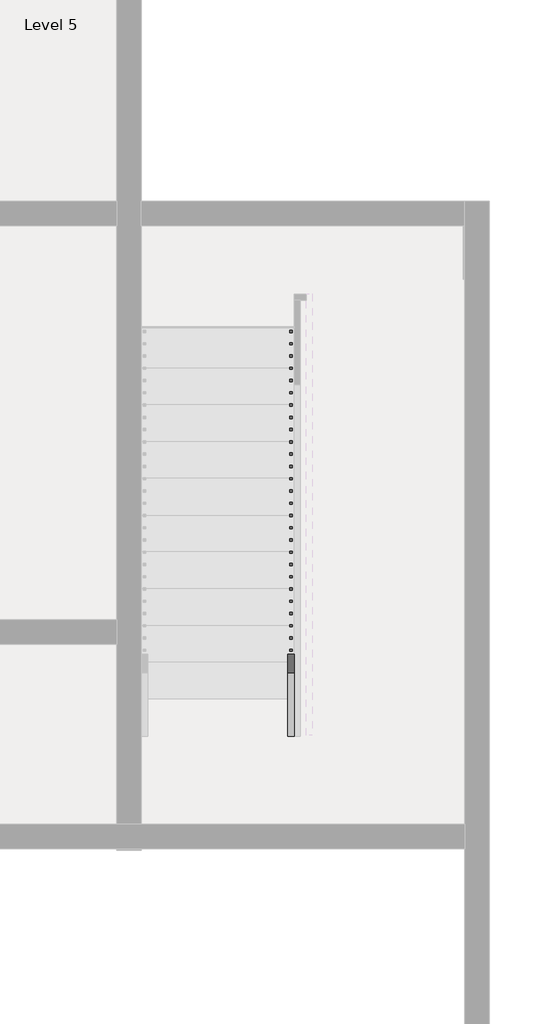
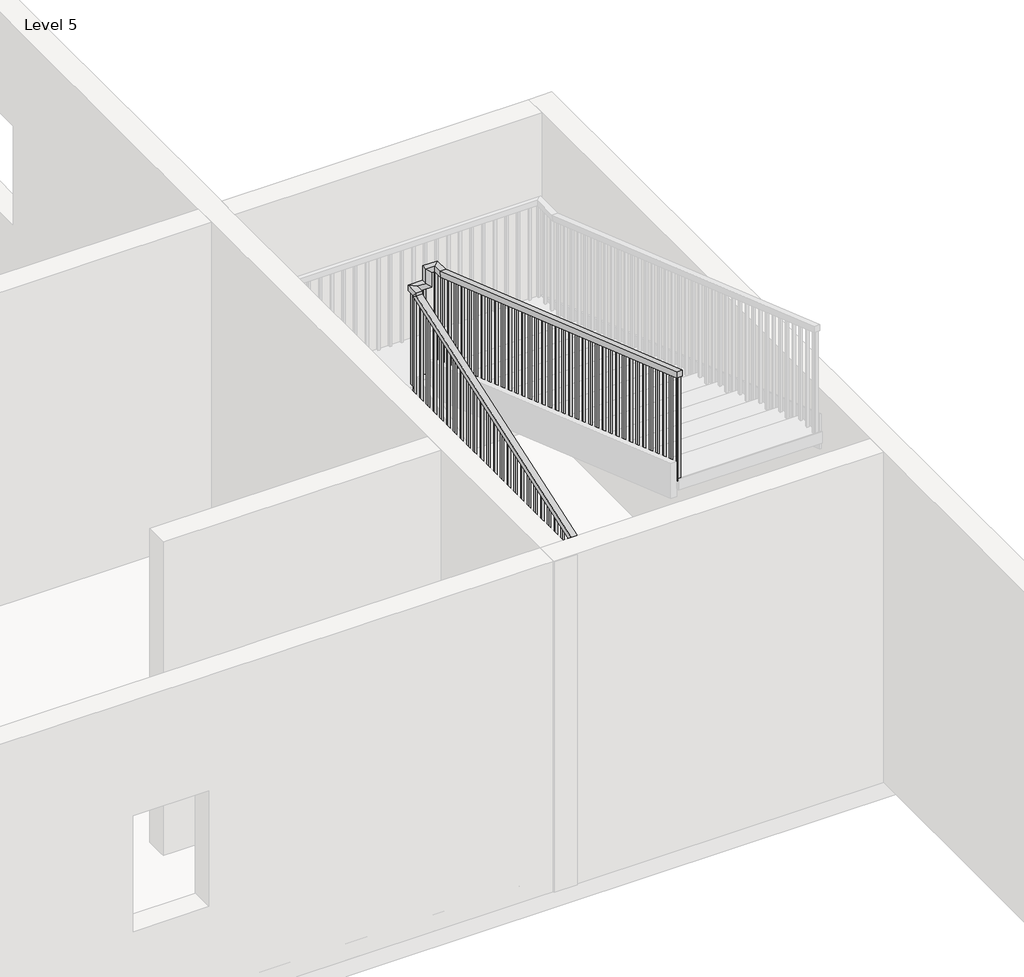
# One storey, part 6 of 14: 1 railing.
"""IFC4 building model written with IfcOpenShell, lengths in millimetres."""

from ifc_helpers import new_model, si_unit, frame, origin, place, context, project, spatial, polyline, outline, extrude, faceted_brep, element, save

model = new_model("IFC4")

# Units and contexts
model_context = context("Model", 3, world=origin())
ifc_project = project(units=[si_unit("LENGTHUNIT", "METRE", prefix="MILLI")], contexts=[model_context])

# Site, building, storey
site = spatial("IfcSite", under=ifc_project)
building = spatial("IfcBuilding", under=site)
storey = spatial("IfcBuildingStorey", under=building, Name="Level 5", Elevation=12192.0)

# Railing
placement = place(None, origin())
element("IfcRailing", 1, ObjectType="Handrail - Rectangular", at=placement, inside=storey, context=model_context, shape_type="SolidModel", body=[
    faceted_brep([(-2644.5381751, -9955.5916506, 13211.9076923), (-2644.5381751, -9955.5916506, 13158.1602476), (-2593.7381751, -9955.5916506, 13158.1602476), (-2593.7381751, -9955.5916506, 13211.9076923), (-2644.5381751, -6367.8416506, 14451.6687908), (-2644.5381751, -6317.0416506, 14415.4754856), (-2593.7381751, -6317.0416506, 14415.4754856), (-2593.7381751, -6367.8416506, 14451.6687908), (-2644.5381751, -6367.8416506, 14478.0), (-2644.5381751, -6317.0416506, 14427.2), (-2593.7381751, -6317.0416506, 14427.2), (-2593.7381751, -6367.8416506, 14478.0), (-2644.5381751, -6240.8416506, 14478.0), (-2644.5381751, -6240.8416506, 14427.2), (-2593.7381751, -6291.6416506, 14427.2), (-2593.7381751, -6291.6416506, 14478.0), (-2517.5381751, -6240.8416506, 14478.0), (-2466.7381751, -6240.8416506, 14427.2), (-2466.7381751, -6291.6416506, 14427.2), (-2517.5381751, -6291.6416506, 14478.0), (-2517.5381751, -6240.8416506, 14609.8846154), (-2466.7381751, -6240.8416506, 14559.0846154), (-2466.7381751, -6291.6416506, 14559.0846154), (-2517.5381751, -6291.6416506, 14609.8846154), (-2390.5381751, -6240.8416506, 14609.8846154), (-2390.5381751, -6240.8416506, 14559.0846154), (-2441.3381751, -6291.6416506, 14559.0846154), (-2441.3381751, -6291.6416506, 14609.8846154), (-2390.5381751, -6367.8416506, 14609.8846154), (-2390.5381751, -6376.3852679, 14559.0846154), (-2441.3381751, -6376.3852679, 14559.0846154), (-2441.3381751, -6367.8416506, 14609.8846154), (-2390.5381751, -9949.2416506, 15849.6), (-2441.3381751, -9949.2416506, 15849.6), (-2441.3381751, -9949.2416506, 15795.842594), (-2390.5381751, -9949.2416506, 15795.842594)], [[[0, 1, 2, 3]], [[1, 0, 4, 5]], [[2, 1, 5, 6]], [[3, 2, 6, 7]], [[0, 3, 7, 4]], [[5, 4, 8, 9]], [[6, 5, 9, 10]], [[7, 6, 10, 11]], [[4, 7, 11, 8]], [[9, 8, 12, 13]], [[10, 9, 13, 14]], [[11, 10, 14, 15]], [[8, 11, 15, 12]], [[13, 12, 16, 17]], [[14, 13, 17, 18]], [[15, 14, 18, 19]], [[12, 15, 19, 16]], [[17, 16, 20, 21]], [[18, 17, 21, 22]], [[19, 18, 22, 23]], [[16, 19, 23, 20]], [[21, 20, 24, 25]], [[22, 21, 25, 26]], [[23, 22, 26, 27]], [[20, 23, 27, 24]], [[25, 24, 28, 29]], [[26, 25, 29, 30]], [[27, 26, 30, 31]], [[24, 27, 31, 28]], [[32, 33, 34, 35]], [[29, 28, 32, 35]], [[30, 29, 35, 34]], [[31, 30, 34, 33]], [[28, 31, 33, 32]]]),
    extrude(outline(polyline([(-9933.3666506, 15790.3474017), (-9914.3166506, 15783.7531709), (-9914.3166506, 14829.6923077), (-9933.3666506, 14829.6923077), (-9933.3666506, 15790.3474017)])), frame((-2425.4631751, 0.0, 0.0), z_axis=(1.0, 0.0, 0.0), x_axis=(0.0, 1.0, 0.0)), (0.0, 0.0, 1.0), 19.05),
    extrude(outline(polyline([(-9831.7666506, 15755.1781709), (-9812.7166506, 15748.5839402), (-9812.7166506, 14829.6923077), (-9831.7666506, 14829.6923077), (-9831.7666506, 15755.1781709)])), frame((-2425.4631751, 0.0, 0.0), z_axis=(1.0, 0.0, 0.0), x_axis=(0.0, 1.0, 0.0)), (0.0, 0.0, 1.0), 19.05),
    extrude(outline(polyline([(-9730.1666506, 15720.0089402), (-9711.1166506, 15713.4147094), (-9711.1166506, 14829.6923077), (-9730.1666506, 14829.6923077), (-9730.1666506, 15720.0089402)])), frame((-2425.4631751, 0.0, 0.0), z_axis=(1.0, 0.0, 0.0), x_axis=(0.0, 1.0, 0.0)), (0.0, 0.0, 1.0), 19.05),
    extrude(outline(polyline([(-9628.5666506, 15684.8397094), (-9609.5166506, 15678.2454786), (-9609.5166506, 14724.1846154), (-9628.5666506, 14724.1846154), (-9628.5666506, 15684.8397094)])), frame((-2425.4631751, 0.0, 0.0), z_axis=(1.0, 0.0, 0.0), x_axis=(0.0, 1.0, 0.0)), (0.0, 0.0, 1.0), 19.05),
    extrude(outline(polyline([(-9526.9666506, 15649.6704786), (-9507.9166506, 15643.0762479), (-9507.9166506, 14724.1846154), (-9526.9666506, 14724.1846154), (-9526.9666506, 15649.6704786)])), frame((-2425.4631751, 0.0, 0.0), z_axis=(1.0, 0.0, 0.0), x_axis=(0.0, 1.0, 0.0)), (0.0, 0.0, 1.0), 19.05),
    extrude(outline(polyline([(-9425.3666506, 15614.5012479), (-9406.3166506, 15607.9070171), (-9406.3166506, 14724.1846154), (-9425.3666506, 14724.1846154), (-9425.3666506, 15614.5012479)])), frame((-2425.4631751, 0.0, 0.0), z_axis=(1.0, 0.0, 0.0), x_axis=(0.0, 1.0, 0.0)), (0.0, 0.0, 1.0), 19.05),
    extrude(outline(polyline([(-9323.7666506, 15579.3320171), (-9304.7166506, 15572.7377863), (-9304.7166506, 14618.6769231), (-9323.7666506, 14618.6769231), (-9323.7666506, 15579.3320171)])), frame((-2425.4631751, 0.0, 0.0), z_axis=(1.0, 0.0, 0.0), x_axis=(0.0, 1.0, 0.0)), (0.0, 0.0, 1.0), 19.05),
    extrude(outline(polyline([(-9222.1666506, 15544.1627863), (-9203.1166506, 15537.5685556), (-9203.1166506, 14618.6769231), (-9222.1666506, 14618.6769231), (-9222.1666506, 15544.1627863)])), frame((-2425.4631751, 0.0, 0.0), z_axis=(1.0, 0.0, 0.0), x_axis=(0.0, 1.0, 0.0)), (0.0, 0.0, 1.0), 19.05),
    extrude(outline(polyline([(-9120.5666506, 15508.9935556), (-9101.5166506, 15502.3993248), (-9101.5166506, 14618.6769231), (-9120.5666506, 14618.6769231), (-9120.5666506, 15508.9935556)])), frame((-2425.4631751, 0.0, 0.0), z_axis=(1.0, 0.0, 0.0), x_axis=(0.0, 1.0, 0.0)), (0.0, 0.0, 1.0), 19.05),
    extrude(outline(polyline([(-9018.9666506, 15473.8243248), (-8999.9166506, 15467.230094), (-8999.9166506, 14513.1692308), (-9018.9666506, 14513.1692308), (-9018.9666506, 15473.8243248)])), frame((-2425.4631751, 0.0, 0.0), z_axis=(1.0, 0.0, 0.0), x_axis=(0.0, 1.0, 0.0)), (0.0, 0.0, 1.0), 19.05),
    extrude(outline(polyline([(-8917.3666506, 15438.655094), (-8898.3166506, 15432.0608632), (-8898.3166506, 14513.1692308), (-8917.3666506, 14513.1692308), (-8917.3666506, 15438.655094)])), frame((-2425.4631751, 0.0, 0.0), z_axis=(1.0, 0.0, 0.0), x_axis=(0.0, 1.0, 0.0)), (0.0, 0.0, 1.0), 19.05),
    extrude(outline(polyline([(-8815.7666506, 15403.4858632), (-8796.7166506, 15396.8916325), (-8796.7166506, 14513.1692308), (-8815.7666506, 14513.1692308), (-8815.7666506, 15403.4858632)])), frame((-2425.4631751, 0.0, 0.0), z_axis=(1.0, 0.0, 0.0), x_axis=(0.0, 1.0, 0.0)), (0.0, 0.0, 1.0), 19.05),
    extrude(outline(polyline([(-8714.1666506, 15368.3166325), (-8695.1166506, 15361.7224017), (-8695.1166506, 14407.6615385), (-8714.1666506, 14407.6615385), (-8714.1666506, 15368.3166325)])), frame((-2425.4631751, 0.0, 0.0), z_axis=(1.0, 0.0, 0.0), x_axis=(0.0, 1.0, 0.0)), (0.0, 0.0, 1.0), 19.05),
    extrude(outline(polyline([(-8612.5666506, 15333.1474017), (-8593.5166506, 15326.5531709), (-8593.5166506, 14407.6615385), (-8612.5666506, 14407.6615385), (-8612.5666506, 15333.1474017)])), frame((-2425.4631751, 0.0, 0.0), z_axis=(1.0, 0.0, 0.0), x_axis=(0.0, 1.0, 0.0)), (0.0, 0.0, 1.0), 19.05),
    extrude(outline(polyline([(-8510.9666506, 15297.9781709), (-8491.9166506, 15291.3839402), (-8491.9166506, 14407.6615385), (-8510.9666506, 14407.6615385), (-8510.9666506, 15297.9781709)])), frame((-2425.4631751, 0.0, 0.0), z_axis=(1.0, 0.0, 0.0), x_axis=(0.0, 1.0, 0.0)), (0.0, 0.0, 1.0), 19.05),
    extrude(outline(polyline([(-8409.3666506, 15262.8089402), (-8390.3166506, 15256.2147094), (-8390.3166506, 14302.1538462), (-8409.3666506, 14302.1538462), (-8409.3666506, 15262.8089402)])), frame((-2425.4631751, 0.0, 0.0), z_axis=(1.0, 0.0, 0.0), x_axis=(0.0, 1.0, 0.0)), (0.0, 0.0, 1.0), 19.05),
    extrude(outline(polyline([(-8307.7666506, 15227.6397094), (-8288.7166506, 15221.0454786), (-8288.7166506, 14302.1538462), (-8307.7666506, 14302.1538462), (-8307.7666506, 15227.6397094)])), frame((-2425.4631751, 0.0, 0.0), z_axis=(1.0, 0.0, 0.0), x_axis=(0.0, 1.0, 0.0)), (0.0, 0.0, 1.0), 19.05),
    extrude(outline(polyline([(-8206.1666506, 15192.4704786), (-8187.1166506, 15185.8762479), (-8187.1166506, 14302.1538462), (-8206.1666506, 14302.1538462), (-8206.1666506, 15192.4704786)])), frame((-2425.4631751, 0.0, 0.0), z_axis=(1.0, 0.0, 0.0), x_axis=(0.0, 1.0, 0.0)), (0.0, 0.0, 1.0), 19.05),
    extrude(outline(polyline([(-8104.5666506, 15157.3012479), (-8085.5166506, 15150.7070171), (-8085.5166506, 14196.6461538), (-8104.5666506, 14196.6461538), (-8104.5666506, 15157.3012479)])), frame((-2425.4631751, 0.0, 0.0), z_axis=(1.0, 0.0, 0.0), x_axis=(0.0, 1.0, 0.0)), (0.0, 0.0, 1.0), 19.05),
    extrude(outline(polyline([(-8002.9666506, 15122.1320171), (-7983.9166506, 15115.5377863), (-7983.9166506, 14196.6461538), (-8002.9666506, 14196.6461538), (-8002.9666506, 15122.1320171)])), frame((-2425.4631751, 0.0, 0.0), z_axis=(1.0, 0.0, 0.0), x_axis=(0.0, 1.0, 0.0)), (0.0, 0.0, 1.0), 19.05),
    extrude(outline(polyline([(-7901.3666506, 15086.9627863), (-7882.3166506, 15080.3685556), (-7882.3166506, 14196.6461538), (-7901.3666506, 14196.6461538), (-7901.3666506, 15086.9627863)])), frame((-2425.4631751, 0.0, 0.0), z_axis=(1.0, 0.0, 0.0), x_axis=(0.0, 1.0, 0.0)), (0.0, 0.0, 1.0), 19.05),
    extrude(outline(polyline([(-7799.7666506, 15051.7935556), (-7780.7166506, 15045.1993248), (-7780.7166506, 14091.1384615), (-7799.7666506, 14091.1384615), (-7799.7666506, 15051.7935556)])), frame((-2425.4631751, 0.0, 0.0), z_axis=(1.0, 0.0, 0.0), x_axis=(0.0, 1.0, 0.0)), (0.0, 0.0, 1.0), 19.05),
    extrude(outline(polyline([(-7698.1666506, 15016.6243248), (-7679.1166506, 15010.030094), (-7679.1166506, 14091.1384615), (-7698.1666506, 14091.1384615), (-7698.1666506, 15016.6243248)])), frame((-2425.4631751, 0.0, 0.0), z_axis=(1.0, 0.0, 0.0), x_axis=(0.0, 1.0, 0.0)), (0.0, 0.0, 1.0), 19.05),
    extrude(outline(polyline([(-7596.5666506, 14981.455094), (-7577.5166506, 14974.8608632), (-7577.5166506, 14091.1384615), (-7596.5666506, 14091.1384615), (-7596.5666506, 14981.455094)])), frame((-2425.4631751, 0.0, 0.0), z_axis=(1.0, 0.0, 0.0), x_axis=(0.0, 1.0, 0.0)), (0.0, 0.0, 1.0), 19.05),
    extrude(outline(polyline([(-7494.9666506, 14946.2858632), (-7475.9166506, 14939.6916325), (-7475.9166506, 13985.6307692), (-7494.9666506, 13985.6307692), (-7494.9666506, 14946.2858632)])), frame((-2425.4631751, 0.0, 0.0), z_axis=(1.0, 0.0, 0.0), x_axis=(0.0, 1.0, 0.0)), (0.0, 0.0, 1.0), 19.05),
    extrude(outline(polyline([(-7393.3666506, 14911.1166325), (-7374.3166506, 14904.5224017), (-7374.3166506, 13985.6307692), (-7393.3666506, 13985.6307692), (-7393.3666506, 14911.1166325)])), frame((-2425.4631751, 0.0, 0.0), z_axis=(1.0, 0.0, 0.0), x_axis=(0.0, 1.0, 0.0)), (0.0, 0.0, 1.0), 19.05),
    extrude(outline(polyline([(-7291.7666506, 14875.9474017), (-7272.7166506, 14869.3531709), (-7272.7166506, 13985.6307692), (-7291.7666506, 13985.6307692), (-7291.7666506, 14875.9474017)])), frame((-2425.4631751, 0.0, 0.0), z_axis=(1.0, 0.0, 0.0), x_axis=(0.0, 1.0, 0.0)), (0.0, 0.0, 1.0), 19.05),
    extrude(outline(polyline([(-7190.1666506, 14840.7781709), (-7171.1166506, 14834.1839402), (-7171.1166506, 13880.1230769), (-7190.1666506, 13880.1230769), (-7190.1666506, 14840.7781709)])), frame((-2425.4631751, 0.0, 0.0), z_axis=(1.0, 0.0, 0.0), x_axis=(0.0, 1.0, 0.0)), (0.0, 0.0, 1.0), 19.05),
    extrude(outline(polyline([(-7088.5666506, 14805.6089402), (-7069.5166506, 14799.0147094), (-7069.5166506, 13880.1230769), (-7088.5666506, 13880.1230769), (-7088.5666506, 14805.6089402)])), frame((-2425.4631751, 0.0, 0.0), z_axis=(1.0, 0.0, 0.0), x_axis=(0.0, 1.0, 0.0)), (0.0, 0.0, 1.0), 19.05),
    extrude(outline(polyline([(-6986.9666506, 14770.4397094), (-6967.9166506, 14763.8454786), (-6967.9166506, 13880.1230769), (-6986.9666506, 13880.1230769), (-6986.9666506, 14770.4397094)])), frame((-2425.4631751, 0.0, 0.0), z_axis=(1.0, 0.0, 0.0), x_axis=(0.0, 1.0, 0.0)), (0.0, 0.0, 1.0), 19.05),
    extrude(outline(polyline([(-6885.3666506, 14735.2704786), (-6866.3166506, 14728.6762479), (-6866.3166506, 13774.6153846), (-6885.3666506, 13774.6153846), (-6885.3666506, 14735.2704786)])), frame((-2425.4631751, 0.0, 0.0), z_axis=(1.0, 0.0, 0.0), x_axis=(0.0, 1.0, 0.0)), (0.0, 0.0, 1.0), 19.05),
    extrude(outline(polyline([(-6783.7666506, 14700.1012479), (-6764.7166506, 14693.5070171), (-6764.7166506, 13774.6153846), (-6783.7666506, 13774.6153846), (-6783.7666506, 14700.1012479)])), frame((-2425.4631751, 0.0, 0.0), z_axis=(1.0, 0.0, 0.0), x_axis=(0.0, 1.0, 0.0)), (0.0, 0.0, 1.0), 19.05),
    extrude(outline(polyline([(-6682.1666506, 14664.9320171), (-6663.1166506, 14658.3377863), (-6663.1166506, 13774.6153846), (-6682.1666506, 13774.6153846), (-6682.1666506, 14664.9320171)])), frame((-2425.4631751, 0.0, 0.0), z_axis=(1.0, 0.0, 0.0), x_axis=(0.0, 1.0, 0.0)), (0.0, 0.0, 1.0), 19.05),
    extrude(outline(polyline([(-6580.5666506, 14629.7627863), (-6561.5166506, 14623.1685556), (-6561.5166506, 13669.1076923), (-6580.5666506, 13669.1076923), (-6580.5666506, 14629.7627863)])), frame((-2425.4631751, 0.0, 0.0), z_axis=(1.0, 0.0, 0.0), x_axis=(0.0, 1.0, 0.0)), (0.0, 0.0, 1.0), 19.05),
    extrude(outline(polyline([(-6478.9666506, 14594.5935556), (-6459.9166506, 14587.9993248), (-6459.9166506, 13669.1076923), (-6478.9666506, 13669.1076923), (-6478.9666506, 14594.5935556)])), frame((-2425.4631751, 0.0, 0.0), z_axis=(1.0, 0.0, 0.0), x_axis=(0.0, 1.0, 0.0)), (0.0, 0.0, 1.0), 19.05),
    extrude(outline(polyline([(-6377.3666506, 14559.4243248), (-6358.3166506, 14552.830094), (-6358.3166506, 13669.1076923), (-6377.3666506, 13669.1076923), (-6377.3666506, 14559.4243248)])), frame((-2425.4631751, 0.0, 0.0), z_axis=(1.0, 0.0, 0.0), x_axis=(0.0, 1.0, 0.0)), (0.0, 0.0, 1.0), 19.05),
    extrude(outline(polyline([(-2527.0631751, -6275.7666506), (-2527.0631751, -6256.7166506), (-2508.0131751, -6256.7166506), (-2508.0131751, -6275.7666506), (-2527.0631751, -6275.7666506)])), frame((0.0, 0.0, 13563.6), z_axis=(0.0, 0.0, 1.0), x_axis=(1.0, 0.0, 0.0)), (0.0, 0.0, 1.0), 863.6),
    extrude(outline(polyline([(-2609.6131751, -6307.5166506), (-2628.6631751, -6307.5166506), (-2628.6631751, -6288.4666506), (-2609.6131751, -6288.4666506), (-2609.6131751, -6307.5166506)])), frame((0.0, 0.0, 13458.0923077), z_axis=(0.0, 0.0, 1.0), x_axis=(1.0, 0.0, 0.0)), (0.0, 0.0, 1.0), 969.1076923),
    extrude(outline(polyline([(-6409.1166506, 14383.6586078), (-6390.0666506, 14390.2414101), (-6390.0666506, 13458.0923077), (-6409.1166506, 13458.0923077), (-6409.1166506, 14383.6586078)])), frame((-2628.6631751, 0.0, 0.0), z_axis=(1.0, 0.0, 0.0), x_axis=(0.0, 1.0, 0.0)), (0.0, 0.0, 1.0), 19.05),
    extrude(outline(polyline([(-6510.7166506, 14348.5503289), (-6491.6666506, 14355.1331312), (-6491.6666506, 13458.0923077), (-6510.7166506, 13458.0923077), (-6510.7166506, 14348.5503289)])), frame((-2628.6631751, 0.0, 0.0), z_axis=(1.0, 0.0, 0.0), x_axis=(0.0, 1.0, 0.0)), (0.0, 0.0, 1.0), 19.05),
    extrude(outline(polyline([(-6612.3166506, 14313.44205), (-6593.2666506, 14320.0248523), (-6593.2666506, 13352.5846154), (-6612.3166506, 13352.5846154), (-6612.3166506, 14313.44205)])), frame((-2628.6631751, 0.0, 0.0), z_axis=(1.0, 0.0, 0.0), x_axis=(0.0, 1.0, 0.0)), (0.0, 0.0, 1.0), 19.05),
    extrude(outline(polyline([(-6713.9166506, 14278.3337711), (-6694.8666506, 14284.9165734), (-6694.8666506, 13352.5846154), (-6713.9166506, 13352.5846154), (-6713.9166506, 14278.3337711)])), frame((-2628.6631751, 0.0, 0.0), z_axis=(1.0, 0.0, 0.0), x_axis=(0.0, 1.0, 0.0)), (0.0, 0.0, 1.0), 19.05),
    extrude(outline(polyline([(-6815.5166506, 14243.2254922), (-6796.4666506, 14249.8082945), (-6796.4666506, 13352.5846154), (-6815.5166506, 13352.5846154), (-6815.5166506, 14243.2254922)])), frame((-2628.6631751, 0.0, 0.0), z_axis=(1.0, 0.0, 0.0), x_axis=(0.0, 1.0, 0.0)), (0.0, 0.0, 1.0), 19.05),
    extrude(outline(polyline([(-6917.1166506, 14208.1172133), (-6898.0666506, 14214.7000156), (-6898.0666506, 13247.0769231), (-6917.1166506, 13247.0769231), (-6917.1166506, 14208.1172133)])), frame((-2628.6631751, 0.0, 0.0), z_axis=(1.0, 0.0, 0.0), x_axis=(0.0, 1.0, 0.0)), (0.0, 0.0, 1.0), 19.05),
    extrude(outline(polyline([(-7018.7166506, 14173.0089344), (-6999.6666506, 14179.5917367), (-6999.6666506, 13247.0769231), (-7018.7166506, 13247.0769231), (-7018.7166506, 14173.0089344)])), frame((-2628.6631751, 0.0, 0.0), z_axis=(1.0, 0.0, 0.0), x_axis=(0.0, 1.0, 0.0)), (0.0, 0.0, 1.0), 19.05),
    extrude(outline(polyline([(-7120.3166506, 14137.9006556), (-7101.2666506, 14144.4834578), (-7101.2666506, 13247.0769231), (-7120.3166506, 13247.0769231), (-7120.3166506, 14137.9006556)])), frame((-2628.6631751, 0.0, 0.0), z_axis=(1.0, 0.0, 0.0), x_axis=(0.0, 1.0, 0.0)), (0.0, 0.0, 1.0), 19.05),
    extrude(outline(polyline([(-7221.9166506, 14102.7923767), (-7202.8666506, 14109.375179), (-7202.8666506, 13141.5692308), (-7221.9166506, 13141.5692308), (-7221.9166506, 14102.7923767)])), frame((-2628.6631751, 0.0, 0.0), z_axis=(1.0, 0.0, 0.0), x_axis=(0.0, 1.0, 0.0)), (0.0, 0.0, 1.0), 19.05),
    extrude(outline(polyline([(-7323.5166506, 14067.6840978), (-7304.4666506, 14074.2669001), (-7304.4666506, 13141.5692308), (-7323.5166506, 13141.5692308), (-7323.5166506, 14067.6840978)])), frame((-2628.6631751, 0.0, 0.0), z_axis=(1.0, 0.0, 0.0), x_axis=(0.0, 1.0, 0.0)), (0.0, 0.0, 1.0), 19.05),
    extrude(outline(polyline([(-7425.1166506, 14032.5758189), (-7406.0666506, 14039.1586212), (-7406.0666506, 13141.5692308), (-7425.1166506, 13141.5692308), (-7425.1166506, 14032.5758189)])), frame((-2628.6631751, 0.0, 0.0), z_axis=(1.0, 0.0, 0.0), x_axis=(0.0, 1.0, 0.0)), (0.0, 0.0, 1.0), 19.05),
    extrude(outline(polyline([(-7526.7166506, 13997.46754), (-7507.6666506, 14004.0503423), (-7507.6666506, 13036.0615385), (-7526.7166506, 13036.0615385), (-7526.7166506, 13997.46754)])), frame((-2628.6631751, 0.0, 0.0), z_axis=(1.0, 0.0, 0.0), x_axis=(0.0, 1.0, 0.0)), (0.0, 0.0, 1.0), 19.05),
    extrude(outline(polyline([(-7628.3166506, 13962.3592611), (-7609.2666506, 13968.9420634), (-7609.2666506, 13036.0615385), (-7628.3166506, 13036.0615385), (-7628.3166506, 13962.3592611)])), frame((-2628.6631751, 0.0, 0.0), z_axis=(1.0, 0.0, 0.0), x_axis=(0.0, 1.0, 0.0)), (0.0, 0.0, 1.0), 19.05),
    extrude(outline(polyline([(-7729.9166506, 13927.2509822), (-7710.8666506, 13933.8337845), (-7710.8666506, 13036.0615385), (-7729.9166506, 13036.0615385), (-7729.9166506, 13927.2509822)])), frame((-2628.6631751, 0.0, 0.0), z_axis=(1.0, 0.0, 0.0), x_axis=(0.0, 1.0, 0.0)), (0.0, 0.0, 1.0), 19.05),
    extrude(outline(polyline([(-7831.5166506, 13892.1427033), (-7812.4666506, 13898.7255056), (-7812.4666506, 12930.5538462), (-7831.5166506, 12930.5538462), (-7831.5166506, 13892.1427033)])), frame((-2628.6631751, 0.0, 0.0), z_axis=(1.0, 0.0, 0.0), x_axis=(0.0, 1.0, 0.0)), (0.0, 0.0, 1.0), 19.05),
    extrude(outline(polyline([(-7933.1166506, 13857.0344244), (-7914.0666506, 13863.6172267), (-7914.0666506, 12930.5538462), (-7933.1166506, 12930.5538462), (-7933.1166506, 13857.0344244)])), frame((-2628.6631751, 0.0, 0.0), z_axis=(1.0, 0.0, 0.0), x_axis=(0.0, 1.0, 0.0)), (0.0, 0.0, 1.0), 19.05),
    extrude(outline(polyline([(-8034.7166506, 13821.9261455), (-8015.6666506, 13828.5089478), (-8015.6666506, 12930.5538462), (-8034.7166506, 12930.5538462), (-8034.7166506, 13821.9261455)])), frame((-2628.6631751, 0.0, 0.0), z_axis=(1.0, 0.0, 0.0), x_axis=(0.0, 1.0, 0.0)), (0.0, 0.0, 1.0), 19.05),
    extrude(outline(polyline([(-8136.3166506, 13786.8178666), (-8117.2666506, 13793.4006689), (-8117.2666506, 12825.0461538), (-8136.3166506, 12825.0461538), (-8136.3166506, 13786.8178666)])), frame((-2628.6631751, 0.0, 0.0), z_axis=(1.0, 0.0, 0.0), x_axis=(0.0, 1.0, 0.0)), (0.0, 0.0, 1.0), 19.05),
    extrude(outline(polyline([(-8237.9166506, 13751.7095877), (-8218.8666506, 13758.29239), (-8218.8666506, 12825.0461538), (-8237.9166506, 12825.0461538), (-8237.9166506, 13751.7095877)])), frame((-2628.6631751, 0.0, 0.0), z_axis=(1.0, 0.0, 0.0), x_axis=(0.0, 1.0, 0.0)), (0.0, 0.0, 1.0), 19.05),
    extrude(outline(polyline([(-8339.5166506, 13716.6013088), (-8320.4666506, 13723.1841111), (-8320.4666506, 12825.0461538), (-8339.5166506, 12825.0461538), (-8339.5166506, 13716.6013088)])), frame((-2628.6631751, 0.0, 0.0), z_axis=(1.0, 0.0, 0.0), x_axis=(0.0, 1.0, 0.0)), (0.0, 0.0, 1.0), 19.05),
    extrude(outline(polyline([(-8441.1166506, 13681.4930299), (-8422.0666506, 13688.0758322), (-8422.0666506, 12719.5384615), (-8441.1166506, 12719.5384615), (-8441.1166506, 13681.4930299)])), frame((-2628.6631751, 0.0, 0.0), z_axis=(1.0, 0.0, 0.0), x_axis=(0.0, 1.0, 0.0)), (0.0, 0.0, 1.0), 19.05),
    extrude(outline(polyline([(-8542.7166506, 13646.384751), (-8523.6666506, 13652.9675533), (-8523.6666506, 12719.5384615), (-8542.7166506, 12719.5384615), (-8542.7166506, 13646.384751)])), frame((-2628.6631751, 0.0, 0.0), z_axis=(1.0, 0.0, 0.0), x_axis=(0.0, 1.0, 0.0)), (0.0, 0.0, 1.0), 19.05),
    extrude(outline(polyline([(-8644.3166506, 13611.2764721), (-8625.2666506, 13617.8592744), (-8625.2666506, 12719.5384615), (-8644.3166506, 12719.5384615), (-8644.3166506, 13611.2764721)])), frame((-2628.6631751, 0.0, 0.0), z_axis=(1.0, 0.0, 0.0), x_axis=(0.0, 1.0, 0.0)), (0.0, 0.0, 1.0), 19.05),
    extrude(outline(polyline([(-8745.9166506, 13576.1681932), (-8726.8666506, 13582.7509955), (-8726.8666506, 12614.0307692), (-8745.9166506, 12614.0307692), (-8745.9166506, 13576.1681932)])), frame((-2628.6631751, 0.0, 0.0), z_axis=(1.0, 0.0, 0.0), x_axis=(0.0, 1.0, 0.0)), (0.0, 0.0, 1.0), 19.05),
    extrude(outline(polyline([(-8847.5166506, 13541.0599143), (-8828.4666506, 13547.6427166), (-8828.4666506, 12614.0307692), (-8847.5166506, 12614.0307692), (-8847.5166506, 13541.0599143)])), frame((-2628.6631751, 0.0, 0.0), z_axis=(1.0, 0.0, 0.0), x_axis=(0.0, 1.0, 0.0)), (0.0, 0.0, 1.0), 19.05),
    extrude(outline(polyline([(-8949.1166506, 13505.9516354), (-8930.0666506, 13512.5344377), (-8930.0666506, 12614.0307692), (-8949.1166506, 12614.0307692), (-8949.1166506, 13505.9516354)])), frame((-2628.6631751, 0.0, 0.0), z_axis=(1.0, 0.0, 0.0), x_axis=(0.0, 1.0, 0.0)), (0.0, 0.0, 1.0), 19.05),
    extrude(outline(polyline([(-9050.7166506, 13470.8433565), (-9031.6666506, 13477.4261588), (-9031.6666506, 12508.5230769), (-9050.7166506, 12508.5230769), (-9050.7166506, 13470.8433565)])), frame((-2628.6631751, 0.0, 0.0), z_axis=(1.0, 0.0, 0.0), x_axis=(0.0, 1.0, 0.0)), (0.0, 0.0, 1.0), 19.05),
    extrude(outline(polyline([(-9152.3166506, 13435.7350776), (-9133.2666506, 13442.3178799), (-9133.2666506, 12508.5230769), (-9152.3166506, 12508.5230769), (-9152.3166506, 13435.7350776)])), frame((-2628.6631751, 0.0, 0.0), z_axis=(1.0, 0.0, 0.0), x_axis=(0.0, 1.0, 0.0)), (0.0, 0.0, 1.0), 19.05),
    extrude(outline(polyline([(-9253.9166506, 13400.6267987), (-9234.8666506, 13407.209601), (-9234.8666506, 12508.5230769), (-9253.9166506, 12508.5230769), (-9253.9166506, 13400.6267987)])), frame((-2628.6631751, 0.0, 0.0), z_axis=(1.0, 0.0, 0.0), x_axis=(0.0, 1.0, 0.0)), (0.0, 0.0, 1.0), 19.05),
    extrude(outline(polyline([(-9355.5166506, 13365.5185198), (-9336.4666506, 13372.1013221), (-9336.4666506, 12403.0153846), (-9355.5166506, 12403.0153846), (-9355.5166506, 13365.5185198)])), frame((-2628.6631751, 0.0, 0.0), z_axis=(1.0, 0.0, 0.0), x_axis=(0.0, 1.0, 0.0)), (0.0, 0.0, 1.0), 19.05),
    extrude(outline(polyline([(-9457.1166506, 13330.4102409), (-9438.0666506, 13336.9930432), (-9438.0666506, 12403.0153846), (-9457.1166506, 12403.0153846), (-9457.1166506, 13330.4102409)])), frame((-2628.6631751, 0.0, 0.0), z_axis=(1.0, 0.0, 0.0), x_axis=(0.0, 1.0, 0.0)), (0.0, 0.0, 1.0), 19.05),
    extrude(outline(polyline([(-9558.7166506, 13295.301962), (-9539.6666506, 13301.8847643), (-9539.6666506, 12403.0153846), (-9558.7166506, 12403.0153846), (-9558.7166506, 13295.301962)])), frame((-2628.6631751, 0.0, 0.0), z_axis=(1.0, 0.0, 0.0), x_axis=(0.0, 1.0, 0.0)), (0.0, 0.0, 1.0), 19.05),
    extrude(outline(polyline([(-9660.3166506, 13260.1936831), (-9641.2666506, 13266.7764854), (-9641.2666506, 12297.5076923), (-9660.3166506, 12297.5076923), (-9660.3166506, 13260.1936831)])), frame((-2628.6631751, 0.0, 0.0), z_axis=(1.0, 0.0, 0.0), x_axis=(0.0, 1.0, 0.0)), (0.0, 0.0, 1.0), 19.05),
    extrude(outline(polyline([(-9761.9166506, 13225.0854043), (-9742.8666506, 13231.6682065), (-9742.8666506, 12297.5076923), (-9761.9166506, 12297.5076923), (-9761.9166506, 13225.0854043)])), frame((-2628.6631751, 0.0, 0.0), z_axis=(1.0, 0.0, 0.0), x_axis=(0.0, 1.0, 0.0)), (0.0, 0.0, 1.0), 19.05),
    extrude(outline(polyline([(-9863.5166506, 13189.9771254), (-9844.4666506, 13196.5599277), (-9844.4666506, 12297.5076923), (-9863.5166506, 12297.5076923), (-9863.5166506, 13189.9771254)])), frame((-2628.6631751, 0.0, 0.0), z_axis=(1.0, 0.0, 0.0), x_axis=(0.0, 1.0, 0.0)), (0.0, 0.0, 1.0), 19.05),
    extrude(outline(polyline([(-2425.4631751, -6275.7666506), (-2425.4631751, -6256.7166506), (-2406.4131751, -6256.7166506), (-2406.4131751, -6275.7666506), (-2425.4631751, -6275.7666506)])), frame((0.0, 0.0, 13563.6), z_axis=(0.0, 0.0, 1.0), x_axis=(1.0, 0.0, 0.0)), (0.0, 0.0, 1.0), 995.4846154),
    extrude(outline(polyline([(-2609.6131751, -6275.7666506), (-2628.6631751, -6275.7666506), (-2628.6631751, -6256.7166506), (-2609.6131751, -6256.7166506), (-2609.6131751, -6275.7666506)])), frame((0.0, 0.0, 13563.6), z_axis=(0.0, 0.0, 1.0), x_axis=(1.0, 0.0, 0.0)), (0.0, 0.0, 1.0), 863.6),
    extrude(outline(polyline([(-9949.2416506, 15795.842594), (-9930.1916506, 15789.2483632), (-9930.1916506, 14829.6923077), (-9949.2416506, 14829.6923077), (-9949.2416506, 15795.842594)])), frame((-2425.4631751, 0.0, 0.0), z_axis=(1.0, 0.0, 0.0), x_axis=(0.0, 1.0, 0.0)), (0.0, 0.0, 1.0), 19.05),
    extrude(outline(polyline([(-9955.5916506, 13158.1602476), (-9936.5416506, 13164.7430499), (-9936.5416506, 12297.5076923), (-9955.5916506, 12297.5076923), (-9955.5916506, 13158.1602476)])), frame((-2628.6631751, 0.0, 0.0), z_axis=(1.0, 0.0, 0.0), x_axis=(0.0, 1.0, 0.0)), (0.0, 0.0, 1.0), 19.05),
])

save(model, "model.ifc")

# Revit data of these elements
# Type "Handrail - Rectangular"
#   Assembly Code = "C2010400"
#   built-in parameter 1008612 = 0.0416667 (stored number, unit not read)
#   built-in parameter 1008611 = 0.0416667 (stored number, unit not read)
#   built-in parameter 1008609 = 0.333333 (stored number, unit not read)
#   built-in parameter 1008604 = 0.166667 (stored number, unit not read)
#   built-in parameter 1008603 = 0.166667 (stored number, unit not read)
#   Railing Height = 3' - 0"
#   built-in parameter 1008630 = 2
#   built-in parameter 1008610 = 2
#   built-in parameter 1008618 = Baluster - Square : 3/4"
# Element 1 (IfcRailing, "Handrail - Rectangular")
#   Phase Created = New Construction
